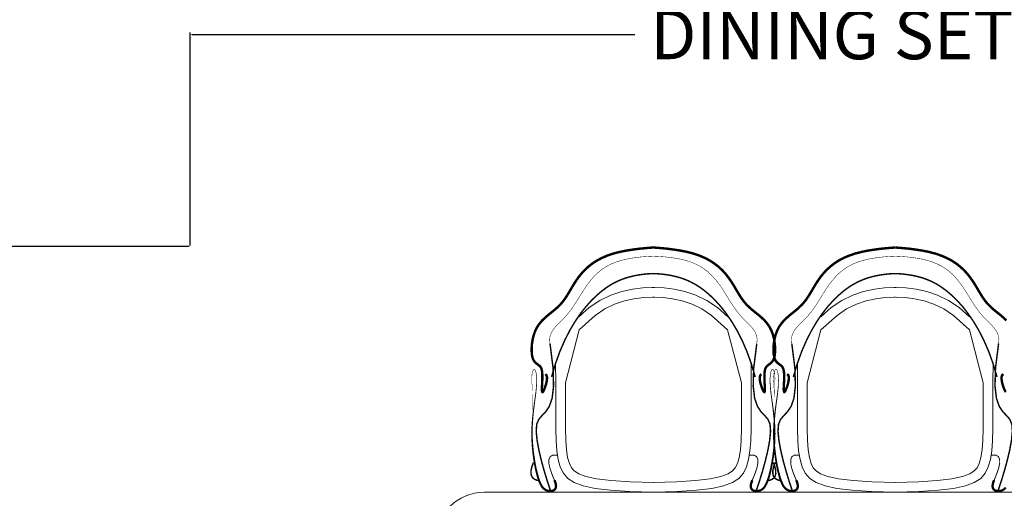
# Model space of a CAD drawing. Units: inches. Extents: x 870 to 1431, y 383 to 1070.
# Tile 5 of 9: x 1091 to 1171, y 718 to 756. Entities that reach past the tile are written whole.
import ezdxf

# ---------------------------------------------------------------- set-up
doc = ezdxf.new("R2010")
doc.units = ezdxf.units.IN
doc.header["$MEASUREMENT"] = 0
doc.layers.add('A-ANNO-DIMS', color=2, linetype='Continuous', lineweight=18)
doc.layers.add('A-FURN', color=8, linetype='Continuous', lineweight=18)
doc.styles.get("Standard").update_dxf_attribs({"font": 'arial.ttf'})
doc.dimstyles.get("Standard").update_dxf_attribs({"dimtxt": 4, "dimasz": 0.18, "dimexe": 0.18, "dimexo": 0.0625, "dimgap": 0.09, "dimtad": 0, "dimtih": 1, "dimtoh": 1, "dimdec": 0, "dimrnd": 6, "dimzin": 0, "dimdsep": 46, "dimlunit": 3, "dimtxsty": 'Standard', "dimcen": 0.09, "dimadec": 0, "dimazin": 0, "dimtfac": 1, "dimtdec": 0, "dimtofl": 0, "dimtmove": 0, "dimatfit": 3, "dimfxl": 1, "dimtolj": 1, "dimtzin": 0, "dimarcsym": 0})

# ---------------------------------------------------------------- blocks, each defined once
blk = doc.blocks.new('ОГ53_на8персон_стол1900х900')
blk.add_line((-850, 279.3), (850, 279.3))
for points, const_width in [([(-723.4, 523.4), (-721.2, 521.4), (-720.1, 518.2), (-719.9, 514.2), (-720.4, 509.6), (-721.4, 504.8), (-722.7, 500.1), (-724.2, 495.7), (-725.7, 492), (-727, 489.2), (-728, 487.3), (-728.9, 486.4), (-729.6, 486.4), (-730.1, 487.3), (-730.4, 489.1), (-730.6, 491.8), (-730.5, 495.4), (-730.3, 499.8), (-730, 504.9), (-729.7, 510.3), (-729.6, 516), (-729.6, 521.5), (-729.9, 526.8), (-730.6, 531.5), (-731.8, 535.5), (-733.5, 538.5), (-735.7, 540.8), (-738.2, 542.8), (-740.8, 544.6), (-743.4, 546.7), (-745.9, 549.3), (-748.1, 552.7), (-749.8, 557.2), (-751.1, 563.1), (-751.7, 570.2), (-751.7, 578.1), (-751, 586.6), (-749.6, 595.4), (-747.4, 604.2), (-744.3, 612.7), (-740.4, 620.6), (-735.5, 627.7), (-730, 634.2), (-723.9, 640.1), (-717.5, 645.6), (-710.9, 650.9), (-704.3, 656.2), (-698.1, 661.7), (-692.2, 667.5), (-686.9, 673.7), (-682.1, 680.3), (-677.6, 687.3), (-673.2, 694.5), (-668.9, 701.9), (-664.4, 709.4), (-659.5, 716.9), (-654.2, 724.4), (-648.3, 731.7), (-641.7, 738.8), (-634.3, 745.6), (-626.1, 752), (-616.9, 758), (-606.7, 763.4), (-595.4, 768.3), (-583, 772.5), (-569.5, 776), (-555.4, 778.8), (-541.5, 780.9), (-528.6, 782.6), (-517.2, 783.7), (-508.2, 784.5), (-502.2, 784.9), (-500, 785)], 5), ([(-276.6, 523.4), (-278.8, 521.4), (-279.9, 518.2), (-280.1, 514.2), (-279.6, 509.6), (-278.6, 504.8), (-277.3, 500.1), (-275.8, 495.7), (-274.3, 492), (-273, 489.2), (-272, 487.3), (-271.1, 486.4), (-270.4, 486.4), (-269.9, 487.3), (-269.6, 489.1), (-269.4, 491.8), (-269.5, 495.4), (-269.7, 499.8), (-270, 504.9), (-270.3, 510.3), (-270.4, 516), (-270.4, 521.5), (-270.1, 526.8), (-269.4, 531.5), (-268.2, 535.5), (-266.5, 538.5), (-264.3, 540.8), (-261.8, 542.8), (-259.2, 544.6), (-256.6, 546.7), (-254.1, 549.3), (-251.9, 552.7), (-250.2, 557.2), (-248.9, 563.1), (-248.3, 570.2), (-248.3, 578.1), (-249, 586.6), (-250.4, 595.4), (-252.6, 604.2), (-255.7, 612.7), (-259.6, 620.6), (-264.5, 627.7), (-270, 634.2), (-276.1, 640.1), (-282.5, 645.6), (-289.1, 650.9), (-295.7, 656.2), (-301.9, 661.7), (-307.8, 667.5), (-313.1, 673.7), (-317.9, 680.3), (-322.4, 687.3), (-326.8, 694.5), (-331.1, 701.9), (-335.6, 709.4), (-340.5, 716.9), (-345.8, 724.4), (-351.7, 731.7), (-358.3, 738.8), (-365.7, 745.6), (-373.9, 752), (-383.1, 758), (-393.3, 763.4), (-404.6, 768.3), (-417, 772.5), (-430.5, 776), (-444.6, 778.8), (-458.5, 780.9), (-471.4, 782.6), (-482.8, 783.7), (-491.8, 784.5), (-497.8, 784.9), (-500, 785)], 5), ([(-223.4, 523.4), (-221.2, 521.4), (-220.1, 518.2), (-219.9, 514.2), (-220.4, 509.6), (-221.4, 504.8), (-222.7, 500.1), (-224.2, 495.7), (-225.7, 492), (-227, 489.2), (-228, 487.3), (-228.9, 486.4), (-229.6, 486.4), (-230.1, 487.3), (-230.4, 489.1), (-230.6, 491.8), (-230.5, 495.4), (-230.3, 499.8), (-230, 504.9), (-229.7, 510.3), (-229.6, 516), (-229.6, 521.5), (-229.9, 526.8), (-230.6, 531.5), (-231.8, 535.5), (-233.5, 538.5), (-235.7, 540.8), (-238.2, 542.8), (-240.8, 544.6), (-243.4, 546.7), (-245.9, 549.3), (-248.1, 552.7), (-249.8, 557.2), (-251.1, 563.1), (-251.7, 570.2), (-251.7, 578.1), (-251, 586.6), (-249.6, 595.4), (-247.4, 604.2), (-244.3, 612.7), (-240.4, 620.6), (-235.5, 627.7), (-230, 634.2), (-223.9, 640.1), (-217.5, 645.6), (-210.9, 650.9), (-204.3, 656.2), (-198.1, 661.7), (-192.2, 667.5), (-186.9, 673.7), (-182.1, 680.3), (-177.6, 687.3), (-173.2, 694.5), (-168.9, 701.9), (-164.4, 709.4), (-159.5, 716.9), (-154.2, 724.4), (-148.3, 731.7), (-141.7, 738.8), (-134.3, 745.6), (-126.1, 752), (-116.9, 758), (-106.7, 763.4), (-95.4, 768.3), (-83, 772.5), (-69.5, 776), (-55.4, 778.8), (-41.5, 780.9), (-28.6, 782.6), (-17.2, 783.7), (-8.2, 784.5), (-2.2, 784.9), (0, 785)], 5), ([(223.4, 523.4), (221.2, 521.4), (220.1, 518.2), (219.9, 514.2), (220.4, 509.6), (221.4, 504.8), (222.7, 500.1), (224.2, 495.7), (225.7, 492), (227, 489.2), (228, 487.3), (228.9, 486.4)], 5), ([(230, 634.2), (223.9, 640.1), (217.5, 645.6), (210.9, 650.9), (204.3, 656.2), (198.1, 661.7), (192.2, 667.5), (186.9, 673.7), (182.1, 680.3), (177.6, 687.3), (173.2, 694.5), (168.9, 701.9), (164.4, 709.4), (159.5, 716.9), (154.2, 724.4), (148.3, 731.7), (141.7, 738.8), (134.3, 745.6), (126.1, 752), (116.9, 758), (106.7, 763.4), (95.4, 768.3), (83, 772.5), (69.5, 776), (55.4, 778.8), (41.5, 780.9), (28.6, 782.6), (17.2, 783.7), (8.2, 784.5), (2.2, 784.9), (0, 785)], 5), ([(-713.8, 586.5), (-714.6, 595.2), (-713.4, 603), (-710.5, 610.1), (-706.3, 616.6), (-701.1, 622.8), (-695.3, 628.7), (-689.3, 634.6), (-683.4, 640.6), (-677.9, 646.8), (-672.8, 653.3), (-667.9, 659.9), (-663.3, 666.7), (-658.8, 673.7), (-654.4, 680.7), (-650, 687.9), (-645.5, 695), (-640.8, 702.2), (-635.8, 709.3), (-630.5, 716.3), (-624.7, 723.1), (-618.5, 729.6), (-611.7, 735.7), (-604.1, 741.4), (-595.9, 746.6), (-586.7, 751.2), (-576.7, 755.2), (-565.5, 758.7), (-553.3, 761.5), (-539.8, 763.8), (-524.9, 765.6), (-508.6, 766.8), (-500, 767.1)], 1), ([(-286.2, 586.5), (-285.4, 595.2), (-286.6, 603), (-289.5, 610.1), (-293.7, 616.6), (-298.9, 622.8), (-304.7, 628.7), (-310.7, 634.6), (-316.6, 640.6), (-322.1, 646.8), (-327.2, 653.3), (-332.1, 659.9), (-336.7, 666.7), (-341.2, 673.7), (-345.6, 680.7), (-350, 687.9), (-354.5, 695), (-359.2, 702.2), (-364.2, 709.3), (-369.5, 716.3), (-375.3, 723.1), (-381.5, 729.6), (-388.3, 735.7), (-395.9, 741.4), (-404.1, 746.6), (-413.3, 751.2), (-423.3, 755.2), (-434.5, 758.7), (-446.7, 761.5), (-460.2, 763.8), (-475.1, 765.6), (-491.4, 766.8), (-500, 767.1)], 1), ([(-213.8, 586.5), (-214.6, 595.2), (-213.4, 603), (-210.5, 610.1), (-206.3, 616.6), (-201.1, 622.8), (-195.3, 628.7), (-189.3, 634.6), (-183.4, 640.6), (-177.9, 646.8), (-172.8, 653.3), (-167.9, 659.9), (-163.3, 666.7), (-158.8, 673.7), (-154.4, 680.7), (-150, 687.9), (-145.5, 695), (-140.8, 702.2), (-135.8, 709.3), (-130.5, 716.3), (-124.7, 723.1), (-118.5, 729.6), (-111.7, 735.7), (-104.1, 741.4), (-95.9, 746.6), (-86.7, 751.2), (-76.7, 755.2), (-65.5, 758.7), (-53.3, 761.5), (-39.8, 763.8), (-24.9, 765.6), (-8.6, 766.8), (0, 767.1)], 1), ([(213.8, 586.5), (214.6, 595.2), (213.4, 603), (210.5, 610.1), (206.3, 616.6), (201.1, 622.8), (195.3, 628.7), (189.3, 634.6), (183.4, 640.6), (177.9, 646.8), (172.8, 653.3), (167.9, 659.9), (163.3, 666.7), (158.8, 673.7), (154.4, 680.7), (150, 687.9), (145.5, 695), (140.8, 702.2), (135.8, 709.3), (130.5, 716.3), (124.7, 723.1), (118.5, 729.6), (111.7, 735.7), (104.1, 741.4), (95.9, 746.6), (86.7, 751.2), (76.7, 755.2), (65.5, 758.7), (53.3, 761.5), (39.8, 763.8), (24.9, 765.6), (8.6, 766.8), (0, 767.1)], 1), ([(-710.6, 517.6), (-702.3, 545.4), (-693.2, 570.7), (-683.2, 593.6), (-672.7, 614.1), (-661.8, 632.4), (-650.6, 648.7), (-639.4, 663), (-628.2, 675.4), (-617.2, 686.1), (-606.5, 695.3), (-596, 703), (-585.8, 709.4), (-575.7, 714.7), (-565.9, 718.9), (-556.4, 722.3), (-547, 724.9), (-537.9, 727), (-529.3, 728.5), (-521.3, 729.6), (-514.3, 730.4), (-508.4, 730.8), (-503.9, 731), (-501, 731.1), (-500, 731.1)], 3), ([(-289.4, 517.6), (-297.7, 545.4), (-306.8, 570.7), (-316.8, 593.6), (-327.3, 614.1), (-338.2, 632.4), (-349.4, 648.7), (-360.6, 663), (-371.8, 675.4), (-382.8, 686.1), (-393.5, 695.3), (-404, 703), (-414.2, 709.4), (-424.3, 714.7), (-434.1, 718.9), (-443.6, 722.3), (-453, 724.9), (-462.1, 727), (-470.7, 728.5), (-478.7, 729.6), (-485.7, 730.4), (-491.6, 730.8), (-496.1, 731), (-499, 731.1), (-500, 731.1)], 3), ([(-210.6, 517.6), (-202.3, 545.4), (-193.2, 570.7), (-183.2, 593.6), (-172.7, 614.1), (-161.8, 632.4), (-150.6, 648.7), (-139.4, 663), (-128.2, 675.4), (-117.2, 686.1), (-106.5, 695.3), (-96, 703), (-85.8, 709.4), (-75.7, 714.7), (-65.9, 718.9), (-56.4, 722.3), (-47, 724.9), (-37.9, 727), (-29.3, 728.5), (-21.3, 729.6), (-14.3, 730.4), (-8.4, 730.8), (-3.9, 731), (-1, 731.1), (0, 731.1)], 3), ([(210.6, 517.6), (202.3, 545.4), (193.2, 570.7), (183.2, 593.6), (172.7, 614.1), (161.8, 632.4), (150.6, 648.7), (139.4, 663), (128.2, 675.4), (117.2, 686.1), (106.5, 695.3), (96, 703), (85.8, 709.4), (75.7, 714.7), (65.9, 718.9), (56.4, 722.3), (47, 724.9), (37.9, 727), (29.3, 728.5), (21.3, 729.6), (14.3, 730.4), (8.4, 730.8), (3.9, 731), (1, 731.1), (0, 731.1)], 3), ([(-713.8, 586.5), (-707.4, 535.5), (-706.4, 498.8), (-709.4, 473.4), (-715.3, 456.6), (-722.6, 445.7), (-730.2, 437.8), (-736.8, 430.2), (-741.2, 420), (-742.3, 405.3), (-740.5, 386.7), (-736.7, 366), (-731.6, 344.5), (-725.9, 323.8), (-720.3, 305.4), (-715.6, 291), (-712.5, 281.9)], 3), ([(-286.2, 586.5), (-292.6, 535.5), (-293.6, 498.8), (-290.6, 473.4), (-284.7, 456.6), (-277.4, 445.7), (-269.8, 437.8), (-263.2, 430.2), (-258.8, 420), (-257.7, 405.3), (-259.5, 386.7), (-263.3, 366), (-268.4, 344.5), (-274.1, 323.8), (-279.7, 305.4), (-284.4, 291), (-287.5, 281.9)], 3), ([(-213.8, 586.5), (-207.4, 535.5), (-206.4, 498.8), (-209.4, 473.4), (-215.3, 456.6), (-222.6, 445.7), (-230.2, 437.8), (-236.8, 430.2), (-241.2, 420), (-242.3, 405.3), (-240.5, 386.7), (-236.7, 366), (-231.6, 344.5), (-225.9, 323.8), (-220.3, 305.4), (-215.6, 291), (-212.5, 281.9)], 3), ([(213.8, 586.5), (207.4, 535.5), (206.4, 498.8), (209.4, 473.4), (215.3, 456.6), (222.6, 445.7), (230.2, 437.8), (236.8, 430.2), (241.2, 420), (242.3, 405.3), (240.5, 386.7), (236.7, 366), (231.6, 344.5), (225.9, 323.8), (220.3, 305.4), (215.6, 291), (212.5, 281.9)], 3), ([(-704.5, 304.2), (-707.8, 312), (-711.3, 321), (-714.3, 330.3), (-716.1, 339.3), (-716, 347.1), (-713.5, 353), (-707.8, 356.1), (-698.2, 355.7)], 2), ([(-295.5, 304.2), (-292.2, 312), (-288.7, 321), (-285.7, 330.3), (-283.9, 339.3), (-284, 347.1), (-286.5, 353), (-292.2, 356.1), (-301.8, 355.7)], 2), ([(-204.5, 304.2), (-207.8, 312), (-211.3, 321), (-214.3, 330.3), (-216.1, 339.3), (-216, 347.1), (-213.5, 353), (-207.8, 356.1), (-198.2, 355.7)], 2), ([(204.5, 304.2), (207.8, 312), (211.3, 321), (214.3, 330.3), (216.1, 339.3), (216, 347.1), (213.5, 353), (207.8, 356.1), (198.2, 355.7)], 2), ([(-748, 341), (-751.3, 331.8), (-753, 324.1), (-753.1, 317.8), (-751.9, 312.9), (-749.4, 309), (-745.8, 306.2), (-741.2, 304.3), (-735.7, 303.1)], 3), ([(-252, 341), (-248.7, 331.8), (-247, 324.1), (-246.9, 317.8), (-248.1, 312.9), (-250.6, 309), (-254.2, 306.2), (-258.8, 304.3), (-264.3, 303.1)], 3), ([(-248, 341), (-251.3, 331.8), (-253, 324.1), (-253.1, 317.8), (-251.9, 312.9), (-249.4, 309), (-245.8, 306.2), (-241.2, 304.3), (-235.7, 303.1)], 3)]:
    blk.add_lwpolyline(points, dxfattribs=dict(const_width=const_width))
for points in [[(-654, 641.6), (-632.6, 660.8), (-610.4, 675.6), (-587.8, 686.5), (-565.2, 694.2), (-543.1, 699), (-522, 701.6), (-502.3, 702.5), (-500, 702.4)], [(-346, 641.6), (-367.4, 660.8), (-389.6, 675.6), (-412.2, 686.5), (-434.8, 694.2), (-456.9, 699), (-478, 701.6), (-497.7, 702.5), (-500, 702.4)], [(-154, 641.6), (-132.6, 660.8), (-110.4, 675.6), (-87.8, 686.5), (-65.2, 694.2), (-43.1, 699), (-22, 701.6), (-2.3, 702.5), (0, 702.4)], [(154, 641.6), (132.6, 660.8), (110.4, 675.6), (87.8, 686.5), (65.2, 694.2), (43.1, 699), (22, 701.6), (2.3, 702.5), (0, 702.4)], [(-653.6, 615), (-620.3, 644.9), (-600.5, 658.2), (-580.2, 668), (-559.8, 674.9), (-539.8, 679.3), (-520.4, 681.7), (-502.1, 682.5), (-500.4, 682.4)], [(-346.4, 615), (-379.7, 644.9), (-399.5, 658.2), (-419.8, 668), (-440.2, 674.9), (-460.2, 679.3), (-479.6, 681.7), (-497.9, 682.5), (-499.6, 682.4)], [(-153.6, 615), (-120.3, 644.9), (-100.5, 658.2), (-80.2, 668), (-59.8, 674.9), (-39.8, 679.3), (-20.4, 681.7), (-2.1, 682.5), (-0.4, 682.4)], [(153.6, 615), (120.3, 644.9), (100.5, 658.2), (80.2, 668), (59.8, 674.9), (39.8, 679.3), (20.4, 681.7), (2.1, 682.5), (0.4, 682.4)], [(-653.6, 615), (-681.9, 505.2), (-681.9, 469.2), (-682, 437.6), (-681.9, 410.1), (-681.2, 386.6), (-679.8, 367), (-677.3, 351.1), (-673.8, 338.8), (-669.4, 329.9), (-663.6, 323.3), (-654.4, 317.4), (-639.5, 311.8), (-617.3, 307), (-587.1, 303.4), (-548.1, 300.9), (-499.4, 299.3)], [(-346.4, 615), (-318.1, 505.2), (-318.1, 469.2), (-318, 437.6), (-318.1, 410.1), (-318.8, 386.6), (-320.2, 367), (-322.7, 351.1), (-326.2, 338.8), (-330.6, 329.9), (-336.4, 323.3), (-345.6, 317.4), (-360.5, 311.8), (-382.7, 307), (-412.9, 303.4), (-451.9, 300.9), (-500.6, 299.3)], [(-153.6, 615), (-181.9, 505.2), (-181.9, 469.2), (-182, 437.6), (-181.9, 410.1), (-181.2, 386.6), (-179.8, 367), (-177.3, 351.1), (-173.8, 338.8), (-169.4, 329.9), (-163.6, 323.3), (-154.4, 317.4), (-139.5, 311.8), (-117.3, 307), (-87.1, 303.4), (-48.1, 300.9), (0.6, 299.3)], [(153.6, 615), (181.9, 505.2), (181.9, 469.2), (182, 437.6), (181.9, 410.1), (181.2, 386.6), (179.8, 367), (177.3, 351.1), (173.8, 338.8), (169.4, 329.9), (163.6, 323.3), (154.4, 317.4), (139.5, 311.8), (117.3, 307), (87.1, 303.4), (48.1, 300.9), (-0.6, 299.3)], [(-702.3, 545.4), (-701.9, 505.1), (-701.9, 469.2), (-702, 437.5), (-701.9, 409.8), (-701.2, 385.6), (-699.6, 364.7), (-696.8, 346.8), (-692.5, 331.5), (-686.1, 318.7), (-676.8, 308), (-663.5, 299.4), (-645.1, 292.5), (-620.6, 287.3), (-589, 283.5), (-549.1, 280.9), (-500, 279.3)], [(-297.7, 545.4), (-298.1, 505.1), (-298.1, 469.2), (-298, 437.5), (-298.1, 409.8), (-298.8, 385.6), (-300.4, 364.7), (-303.2, 346.8), (-307.5, 331.5), (-313.9, 318.7), (-323.2, 308), (-336.5, 299.4), (-354.9, 292.5), (-379.4, 287.3), (-411, 283.5), (-450.9, 280.9), (-500, 279.3)], [(-202.3, 545.4), (-201.9, 505.1), (-201.9, 469.2), (-202, 437.5), (-201.9, 409.8), (-201.2, 385.6), (-199.6, 364.7), (-196.8, 346.8), (-192.5, 331.5), (-186.1, 318.7), (-176.8, 308), (-163.5, 299.4), (-145.1, 292.5), (-120.6, 287.3), (-89, 283.5), (-49.1, 280.9), (0, 279.3)], [(202.3, 545.4), (201.9, 505.1), (201.9, 469.2), (202, 437.5), (201.9, 409.8), (201.2, 385.6), (199.6, 364.7), (196.8, 346.8), (192.5, 331.5), (186.1, 318.7), (176.8, 308), (163.5, 299.4), (145.1, 292.5), (120.6, 287.3), (89, 283.5), (49.1, 280.9), (0, 279.3)]]:
    blk.add_lwpolyline(points)
for points in [[(-704.5, 304.2, 5, 4.91, 0), (-702, 297.4, 4.91, 4.84, 0), (-701.3, 292.1, 4.84, 4.78, 0), (-701.9, 288.1, 4.78, 4.74, 0), (-703.7, 285.1, 4.74, 4.7, 0), (-706.3, 283.2, 4.7, 4.65, 0), (-709.4, 282.2, 4.65, 4.61, 0), (-712.9, 281.8, 4.61, 4.56, 0), (-716.5, 282.1, 4.56, 4.52, 0), (-719.8, 282.8, 4.52, 4.47, 0), (-722.9, 284.1, 4.47, 4.43, 0), (-725.9, 286.1, 4.43, 4.38, 0), (-728.7, 288.8, 4.38, 4.32, 0), (-731.3, 292.5, 4.32, 4.25, 0), (-733.8, 297.3, 4.25, 4.17, 0), (-736.3, 303.2, 4.17, 4.07, 0), (-738.7, 310.4, 4.07, 3.95, 0), (-741, 318.9, 3.95, 3.82, 0), (-743.3, 328.7, 3.82, 3.68, 0), (-745.4, 339.4, 3.68, 3.53, 0), (-747.2, 350.9, 3.53, 3.37, 0), (-748.8, 363, 3.37, 3.21, 0), (-750, 375.5, 3.21, 3.05, 0), (-750.8, 388.2, 3.05, 2.88, 0), (-751.1, 400.7, 2.88, 2.72, 0), (-750.9, 413.1, 2.72, 2.57, 0), (-750.2, 425.1, 2.57, 2.41, 0), (-749.2, 436.7, 2.41, 2.27, 0), (-748, 447.8, 2.27, 2.13, 0), (-746.7, 458.3, 2.13, 2, 0), (-745.3, 468.2, 2, 1.88, 0), (-744.1, 477.3, 1.88, 1.78, 0), (-743, 485.6, 1.78, 1.68, 0), (-742.2, 493.1, 1.68, 1.59, 0), (-741.7, 499.6, 1.59, 1.52, 0), (-741.4, 505.4, 1.52, 1.45, 0), (-741.3, 510.5, 1.45, 1.4, 0), (-741.4, 514.9, 1.4, 1.35, 0), (-741.6, 518.7, 1.35, 1.3, 0), (-742, 521.9, 1.3, 1.27, 0), (-742.4, 524.7, 1.27, 1.24, 0), (-742.8, 527, 1.24, 1.21, 0), (-743.3, 528.8, 1.21, 1.19, 0), (-743.8, 530.3, 1.19, 1.18, 0), (-744.3, 531.5, 1.18, 1.16, 0), (-744.8, 532.3, 1.16, 1.15, 0), (-745.3, 532.9, 1.15, 1.14, 0), (-745.8, 533.2, 1.14, 1.14, 0), (-746.3, 533.3, 1.14, 1.13, 0), (-746.8, 533.2, 1.13, 1.12, 0), (-747.3, 533, 1.12, 1.12, 0), (-747.8, 532.5, 1.12, 1.11, 0), (-748.3, 531.9, 1.11, 1.09, 0), (-748.7, 531.1, 1.09, 1.08, 0), (-749.1, 530.2, 1.08, 1.07, 0), (-749.5, 529.1, 1.07, 1.05, 0), (-749.9, 527.9, 1.05, 1.03, 0), (-750.3, 526.5, 1.03, 1.01, 0), (-750.6, 524.9, 1.01, 0.986, 0), (-750.9, 523.1, 0.986, 0.959, 0), (-751.1, 521, 0.959, 0.926, 0), (-751.3, 518.5, 0.926, 0.889, 0), (-751.4, 515.7, 0.889, 0.846, 0), (-751.4, 512.3, 0.846, 0.796, 0), (-751.3, 508.5, 0.796, 0.738, 0), (-751.1, 504, 0.738, 0.672, 0), (-750.8, 498.9, 0.672, 0.595, 0), (-750.6, 493, 0.595, 0.506, 0), (-750.3, 486.1, 0.506, 0.404, 0), (-750.1, 478.2, 0.404, 0.286, 0), (-749.9, 469.2, 0.286, 0.152, 0), (-749.9, 458.8, 0.152, 0, 0), (-750, 447.1, 0, 0, 0)], [(-295.5, 304.2, 5, 4.91, 0), (-298, 297.4, 4.91, 4.84, 0), (-298.7, 292.1, 4.84, 4.78, 0), (-298.1, 288.1, 4.78, 4.74, 0), (-296.3, 285.1, 4.74, 4.7, 0), (-293.7, 283.2, 4.7, 4.65, 0), (-290.6, 282.2, 4.65, 4.61, 0), (-287.1, 281.8, 4.61, 4.56, 0), (-283.5, 282.1, 4.56, 4.52, 0), (-280.2, 282.8, 4.52, 4.47, 0), (-277.1, 284.1, 4.47, 4.43, 0), (-274.1, 286.1, 4.43, 4.38, 0), (-271.3, 288.8, 4.38, 4.32, 0), (-268.7, 292.5, 4.32, 4.25, 0), (-266.2, 297.3, 4.25, 4.17, 0), (-263.7, 303.2, 4.17, 4.07, 0), (-261.3, 310.4, 4.07, 3.95, 0), (-259, 318.9, 3.95, 3.82, 0), (-256.7, 328.7, 3.82, 3.68, 0), (-254.6, 339.4, 3.68, 3.53, 0), (-252.8, 350.9, 3.53, 3.37, 0), (-251.2, 363, 3.37, 3.21, 0), (-250, 375.5, 3.21, 3.05, 0), (-249.2, 388.2, 3.05, 2.88, 0), (-248.9, 400.7, 2.88, 2.72, 0), (-249.1, 413.1, 2.72, 2.57, 0), (-249.8, 425.1, 2.57, 2.41, 0), (-250.8, 436.7, 2.41, 2.27, 0), (-252, 447.8, 2.27, 2.13, 0), (-253.3, 458.3, 2.13, 2, 0), (-254.7, 468.2, 2, 1.88, 0), (-255.9, 477.3, 1.88, 1.78, 0), (-257, 485.6, 1.78, 1.68, 0), (-257.8, 493.1, 1.68, 1.59, 0), (-258.3, 499.6, 1.59, 1.52, 0), (-258.6, 505.4, 1.52, 1.45, 0), (-258.7, 510.5, 1.45, 1.4, 0), (-258.6, 514.9, 1.4, 1.35, 0), (-258.4, 518.7, 1.35, 1.3, 0), (-258, 521.9, 1.3, 1.27, 0), (-257.6, 524.7, 1.27, 1.24, 0), (-257.2, 527, 1.24, 1.21, 0), (-256.7, 528.8, 1.21, 1.19, 0), (-256.2, 530.3, 1.19, 1.18, 0), (-255.7, 531.5, 1.18, 1.16, 0), (-255.2, 532.3, 1.16, 1.15, 0), (-254.7, 532.9, 1.15, 1.14, 0), (-254.2, 533.2, 1.14, 1.14, 0), (-253.7, 533.3, 1.14, 1.13, 0), (-253.2, 533.2, 1.13, 1.12, 0), (-252.7, 533, 1.12, 1.12, 0), (-252.2, 532.5, 1.12, 1.11, 0), (-251.7, 531.9, 1.11, 1.09, 0), (-251.3, 531.1, 1.09, 1.08, 0), (-250.9, 530.2, 1.08, 1.07, 0), (-250.5, 529.1, 1.07, 1.05, 0), (-250.1, 527.9, 1.05, 1.03, 0), (-249.7, 526.5, 1.03, 1.01, 0), (-249.4, 524.9, 1.01, 0.986, 0), (-249.1, 523.1, 0.986, 0.959, 0), (-248.9, 521, 0.959, 0.926, 0), (-248.7, 518.5, 0.926, 0.889, 0), (-248.6, 515.7, 0.889, 0.846, 0), (-248.6, 512.3, 0.846, 0.796, 0), (-248.7, 508.5, 0.796, 0.738, 0), (-248.9, 504, 0.738, 0.672, 0), (-249.2, 498.9, 0.672, 0.595, 0), (-249.4, 493, 0.595, 0.506, 0), (-249.7, 486.1, 0.506, 0.404, 0), (-249.9, 478.2, 0.404, 0.286, 0), (-250.1, 469.2, 0.286, 0.152, 0), (-250.1, 458.8, 0.152, 0, 0), (-250, 447.1, 0, 0, 0)], [(-204.5, 304.2, 5, 4.91, 0), (-202, 297.4, 4.91, 4.84, 0), (-201.3, 292.1, 4.84, 4.78, 0), (-201.9, 288.1, 4.78, 4.74, 0), (-203.7, 285.1, 4.74, 4.7, 0), (-206.3, 283.2, 4.7, 4.65, 0), (-209.4, 282.2, 4.65, 4.61, 0), (-212.9, 281.8, 4.61, 4.56, 0), (-216.5, 282.1, 4.56, 4.52, 0), (-219.8, 282.8, 4.52, 4.47, 0), (-222.9, 284.1, 4.47, 4.43, 0), (-225.9, 286.1, 4.43, 4.38, 0), (-228.7, 288.8, 4.38, 4.32, 0), (-231.3, 292.5, 4.32, 4.25, 0), (-233.8, 297.3, 4.25, 4.17, 0), (-236.3, 303.2, 4.17, 4.07, 0), (-238.7, 310.4, 4.07, 3.95, 0), (-241, 318.9, 3.95, 3.82, 0), (-243.3, 328.7, 3.82, 3.68, 0), (-245.4, 339.4, 3.68, 3.53, 0), (-247.2, 350.9, 3.53, 3.37, 0), (-248.8, 363, 3.37, 3.21, 0), (-250, 375.5, 3.21, 3.05, 0), (-250.8, 388.2, 3.05, 2.88, 0), (-251.1, 400.7, 2.88, 2.72, 0), (-250.9, 413.1, 2.72, 2.57, 0), (-250.2, 425.1, 2.57, 2.41, 0), (-249.2, 436.7, 2.41, 2.27, 0), (-248, 447.8, 2.27, 2.13, 0), (-246.7, 458.3, 2.13, 2, 0), (-245.3, 468.2, 2, 1.88, 0), (-244.1, 477.3, 1.88, 1.78, 0), (-243, 485.6, 1.78, 1.68, 0), (-242.2, 493.1, 1.68, 1.59, 0), (-241.7, 499.6, 1.59, 1.52, 0), (-241.4, 505.4, 1.52, 1.45, 0), (-241.3, 510.5, 1.45, 1.4, 0), (-241.4, 514.9, 1.4, 1.35, 0), (-241.6, 518.7, 1.35, 1.3, 0), (-242, 521.9, 1.3, 1.27, 0), (-242.4, 524.7, 1.27, 1.24, 0), (-242.8, 527, 1.24, 1.21, 0), (-243.3, 528.8, 1.21, 1.19, 0), (-243.8, 530.3, 1.19, 1.18, 0), (-244.3, 531.5, 1.18, 1.16, 0), (-244.8, 532.3, 1.16, 1.15, 0), (-245.3, 532.9, 1.15, 1.14, 0), (-245.8, 533.2, 1.14, 1.14, 0), (-246.3, 533.3, 1.14, 1.13, 0), (-246.8, 533.2, 1.13, 1.12, 0), (-247.3, 533, 1.12, 1.12, 0), (-247.8, 532.5, 1.12, 1.11, 0), (-248.3, 531.9, 1.11, 1.09, 0), (-248.7, 531.1, 1.09, 1.08, 0), (-249.1, 530.2, 1.08, 1.07, 0), (-249.5, 529.1, 1.07, 1.05, 0), (-249.9, 527.9, 1.05, 1.03, 0), (-250.3, 526.5, 1.03, 1.01, 0), (-250.6, 524.9, 1.01, 0.986, 0), (-250.9, 523.1, 0.986, 0.959, 0), (-251.1, 521, 0.959, 0.926, 0), (-251.3, 518.5, 0.926, 0.889, 0), (-251.4, 515.7, 0.889, 0.846, 0), (-251.4, 512.3, 0.846, 0.796, 0), (-251.3, 508.5, 0.796, 0.738, 0), (-251.1, 504, 0.738, 0.672, 0), (-250.8, 498.9, 0.672, 0.595, 0), (-250.6, 493, 0.595, 0.506, 0), (-250.3, 486.1, 0.506, 0.404, 0), (-250.1, 478.2, 0.404, 0.286, 0), (-249.9, 469.2, 0.286, 0.152, 0), (-249.9, 458.8, 0.152, 0, 0), (-250, 447.1, 0, 0, 0)], [(204.5, 304.2, 5, 4.91, 0), (202, 297.4, 4.91, 4.84, 0), (201.3, 292.1, 4.84, 4.78, 0), (201.9, 288.1, 4.78, 4.74, 0), (203.7, 285.1, 4.74, 4.7, 0), (206.3, 283.2, 4.7, 4.65, 0), (209.4, 282.2, 4.65, 4.61, 0), (212.9, 281.8, 4.61, 4.56, 0), (216.5, 282.1, 4.56, 4.52, 0), (219.8, 282.8, 4.52, 4.47, 0), (222.9, 284.1, 4.47, 4.43, 0), (225.9, 286.1, 4.43, 4.38, 0), (228.7, 288.8, 4.38, 4.32, 0)]]:
    blk.add_lwpolyline(points, format="xyseb")
blk.add_arc((-850, 179.3), 100, 90, 180)
blk = doc.blocks.new('*D123')
at = {"layer": 'A-ANNO-DIMS', "color": 0, "lineweight": -2, "transparency": 16777216}
for p, q in [((1104.966, 738.101), (1104.966, 755.441)), ((1105.146, 755.261), (1141.184, 755.261)), ((1219.601, 755.261), (1183.563, 755.261)), ((1219.781, 738.101), (1219.781, 755.441))]:
    blk.add_line(p, q, dxfattribs=at)
at = {"layer": 'A-ANNO-DIMS', "color": 0, "transparency": 16777216}
for points in [[(1105.146, 755.291), (1105.146, 755.231), (1104.966, 755.261)], [(1219.601, 755.291), (1219.601, 755.231), (1219.781, 755.261)]]:
    blk.add_solid(points, dxfattribs=at)
at = {"layer": 'Defpoints', "color": 0, "transparency": 16777216}
for p in [(1219.781, 755.261), (1104.966, 738.039), (1219.781, 738.039)]:
    blk.add_point(p, dxfattribs=at)
at = {"layer": 'A-ANNO-DIMS', "color": 0, "transparency": 16777216, "insert": (1162.373, 755.261), "char_height": 4, "attachment_point": 5}
blk.add_mtext('\\A1;DINING SET 115', dxfattribs=at)
blk = doc.blocks.new('*D124')
at = {"layer": 'A-ANNO-DIMS', "color": 0, "lineweight": -2, "transparency": 16777216}
for p, q in [((1104.903, 738.039), (1087.564, 738.039)), ((1087.744, 737.859), (1087.744, 702.44)), ((1087.744, 662.774), (1087.744, 698.192)), ((1104.903, 662.594), (1087.564, 662.594))]:
    blk.add_line(p, q, dxfattribs=at)
at = {"layer": 'A-ANNO-DIMS', "color": 0, "transparency": 16777216}
for points in [[(1087.714, 737.859), (1087.774, 737.859), (1087.744, 738.039)], [(1087.714, 662.774), (1087.774, 662.774), (1087.744, 662.594)]]:
    blk.add_solid(points, dxfattribs=at)
at = {"layer": 'Defpoints', "color": 0, "transparency": 16777216}
for p in [(1087.744, 738.039), (1104.966, 738.039), (1104.966, 662.594)]:
    blk.add_point(p, dxfattribs=at)
at = {"layer": 'A-ANNO-DIMS', "color": 0, "transparency": 16777216, "insert": (1087.744, 700.316), "char_height": 4, "attachment_point": 5}
blk.add_mtext('\\A1;75', dxfattribs=at)
blk = doc.blocks.new('*D126')
at = {"layer": 'A-ANNO-DIMS', "color": 0, "lineweight": -2, "transparency": 16777216}
for p, q in [((1168.728, 1009.477), (876.241, 1009.477)), ((876.421, 1009.297), (876.421, 715.166)), ((876.421, 416.77), (876.421, 710.901)), ((1094.634, 416.59), (876.241, 416.59))]:
    blk.add_line(p, q, dxfattribs=at)
at = {"layer": 'A-ANNO-DIMS', "color": 0, "transparency": 16777216}
for points in [[(876.391, 1009.297), (876.451, 1009.297), (876.421, 1009.477)], [(876.391, 416.77), (876.451, 416.77), (876.421, 416.59)]]:
    blk.add_solid(points, dxfattribs=at)
at = {"layer": 'Defpoints', "color": 0, "transparency": 16777216}
for p in [(876.421, 1009.477), (1168.791, 1009.477), (1094.697, 416.59)]:
    blk.add_point(p, dxfattribs=at)
at = {"layer": 'A-ANNO-DIMS', "color": 0, "transparency": 16777216, "insert": (876.421, 713.034), "char_height": 4, "attachment_point": 5}
blk.add_mtext('\\A1;592.9', dxfattribs=at)

msp = doc.modelspace()

# ---------------------------------------------------------------- block references
at = {"layer": 'A-FURN', "xscale": 0.0393700787401575, "yscale": 0.0393700787401575, "zscale": 0.0393700787401575}
msp.add_blockref('ОГ53_на8персон_стол1900х900', (1162.3732, 707.036), dxfattribs=at)

# ---------------------------------------------------------------- dimensions: what is measured, and where the dimension line sits
at = {"layer": 'A-ANNO-DIMS'}
for base, p1, p2, override, picture, middle in [((876.4215, 1009.4772), (1094.6967, 416.59), (1168.7907, 1009.4772), {"dimdec": 1, "dimlfac": 1, "dimrnd": 0, "dimzin": 0, "dimdsep": 46, "dimlunit": 2}, '*D126', (876.4215, 713.0336)), ((1087.7437, 738.0387), (1104.9659, 662.594), (1104.9659, 738.0387), {"dimdec": 0, "dimlfac": 1, "dimrnd": 0, "dimzin": 0, "dimdsep": 46, "dimlunit": 2}, '*D124', (1087.7437, 700.3164))]:
    dim = msp.add_linear_dim(base=base, p1=p1, p2=p2, angle=90, dimstyle='Standard', override=override, dxfattribs=at)
    dim.commit()
    dim.dimension.update_dxf_attribs({"geometry": picture, "text_midpoint": middle})
dim = msp.add_linear_dim(base=(1219.7806, 755.2609), p1=(1104.9659, 738.0387), p2=(1219.7806, 738.0387), text='DINING SET <>', dimstyle='Standard', override={"dimdec": 0, "dimlfac": 1, "dimrnd": 0, "dimzin": 0, "dimdsep": 46, "dimlunit": 2}, dxfattribs=at)
dim.commit()
dim.dimension.update_dxf_attribs({"geometry": '*D123', "text_midpoint": (1162.3732, 755.2609)})

doc.saveas('drawing.dxf')
